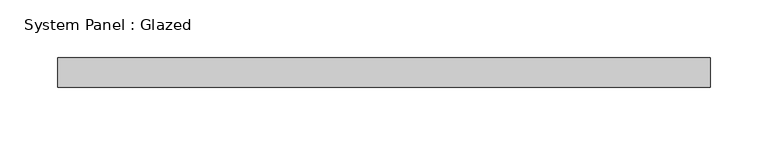
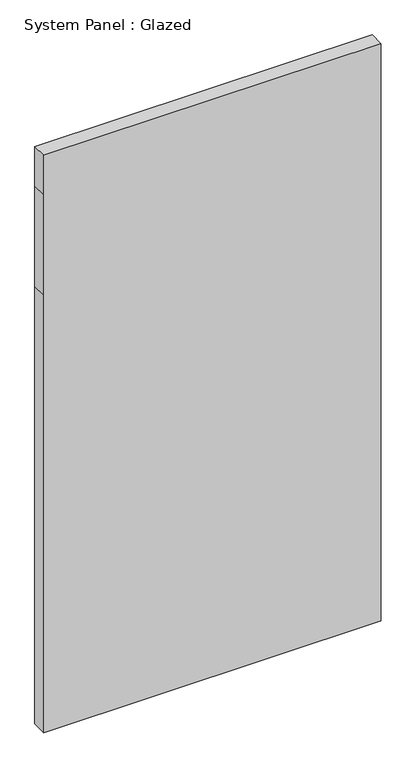
"""IFC4 building model written with IfcOpenShell, lengths in millimetres: plate geometry, System Panel : Glazed."""

from ifc_helpers import new_model, si_unit, frame, origin, place, context, project, spatial, polyline, outline, extrude, source, transform, mapped, element, save


def system_panel_glazed_4710a741(model_context):
    return source(origin(), model_context, "Body", "SweptSolid", [
        extrude(outline(polyline([(0.0, -282.575), (0.0, 282.575), (774.7, 282.575), (952.5, 282.575), (1022.35, 282.575), (1022.35, -282.575), (952.5, -282.575), (774.7, -282.575), (0.0, -282.575)])), frame((0.0, 19.05, 0.0), z_axis=(0.0, 1.0, 0.0), x_axis=(0.0, 0.0, 1.0)), (0.0, 0.0, 1.0), 25.4),
    ])


if __name__ == "__main__":
    model = new_model("IFC4")
    model_context = context("Model", 3, world=origin())
    ifc_project = project(units=[si_unit("LENGTHUNIT", "METRE", prefix="MILLI")], contexts=[model_context])
    site = spatial("IfcSite", under=ifc_project)
    building = spatial("IfcBuilding", under=site)
    placement = place(None, origin())
    system_panel_glazed_shape = system_panel_glazed_4710a741(model_context)
    element("IfcPlate", 1, ObjectType="System Panel : Glazed", at=placement, inside=building, context=model_context, shape_type="MappedRepresentation", body=[
        mapped(system_panel_glazed_shape, transform((0.0, 0.0, 0.0), x_axis=(1.0, 0.0, 0.0), y_axis=(0.0, 1.0, 0.0), z_axis=(0.0, 0.0, 1.0))),
    ])
    save(model, "model.ifc")

# Revit data of these elements
# Type "System Panel : Glazed"
#   Construction Type Id = "GSP4R"
#   Analytic Construction = "1/8 in Pilkington single glazing"
#   Visual Light Transmittance = 0.9
#   Solar Heat Gain Coefficient = 0.86
#   Heat Transfer Coefficient (U) = 1.18115 BTU/(h·ft²·°F)
#   Define Thermal Properties by = 1
# Element 1 (IfcPlate, "System Panel : Glazed")
#   Materials on its faces: "Glass"
# Materials
#   "Glass": class "Glass", colour RGB 0 128 192, transparency 0.75, Description = "Soda Lime Glass", Cost = 0
